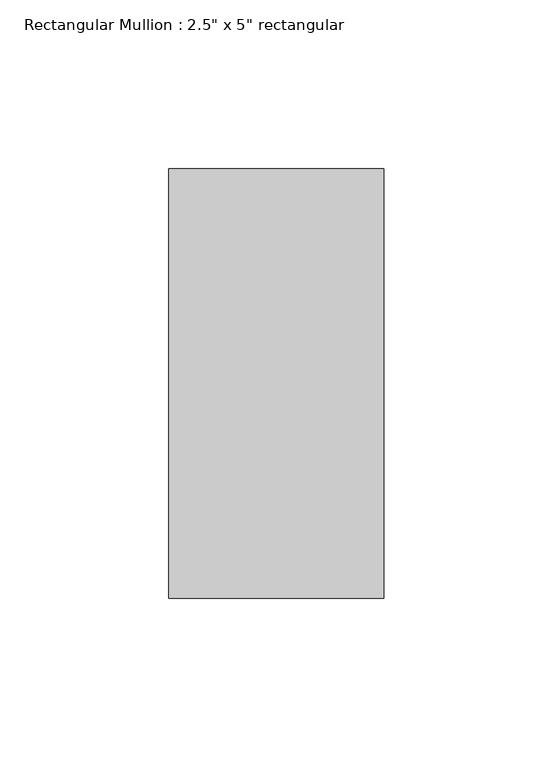
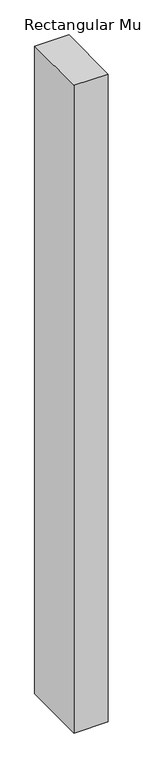
"""IFC4 building model written with IfcOpenShell, lengths in millimetres: member geometry."""

from ifc_helpers import new_model, si_unit, frame, origin, place, context, project, spatial, polyline, outline, extrude, source, transform, mapped, element, save


def member_8dd6731c(model_context):
    return source(origin(), model_context, "Body", "SweptSolid", [
        extrude(outline(polyline([(31.75, 63.5), (31.75, -63.5), (-31.75, -63.5), (-31.75, 63.5), (31.75, 63.5)])), frame((0.0, 0.0, -1273.4060005), z_axis=(0.0, 0.0, 1.0), x_axis=(1.0, 0.0, 0.0)), (0.0, 0.0, 1.0), 1273.4060005),
    ])


if __name__ == "__main__":
    model = new_model("IFC4")
    model_context = context("Model", 3, world=origin())
    ifc_project = project(units=[si_unit("LENGTHUNIT", "METRE", prefix="MILLI")], contexts=[model_context])
    site = spatial("IfcSite", under=ifc_project)
    building = spatial("IfcBuilding", under=site)
    placement = place(None, origin())
    member_shape = member_8dd6731c(model_context)
    element("IfcMember", 1, ObjectType="Rectangular Mullion : 2.5\" x 5\" rectangular", at=placement, inside=building, context=model_context, shape_type="MappedRepresentation", body=[
        mapped(member_shape, transform((0.0, 0.0, 0.0), x_axis=(1.0, 0.0, 0.0), y_axis=(0.0, 1.0, 0.0), z_axis=(0.0, 0.0, 1.0))),
    ])
    save(model, "model.ifc")

# Revit data of these elements
# Type "Rectangular Mullion : 2.5\" x 5\" rectangular"
#   built-in parameter 1007304 = 0.416667 (stored number, unit not read)
#   built-in parameter 1007301 = 0.104167 (stored number, unit not read)
#   built-in parameter 1007300 = 0.104167 (stored number, unit not read)
# Element 1 (IfcMember, "Rectangular Mullion : 2.5\" x 5\" rectangular")
#   Materials on its faces: "Aluminum"
# Materials
#   "Aluminum": class "Metal", colour RGB 247 247 247, transparency 0, Description = "Aluminum 6061", Cost = 0
